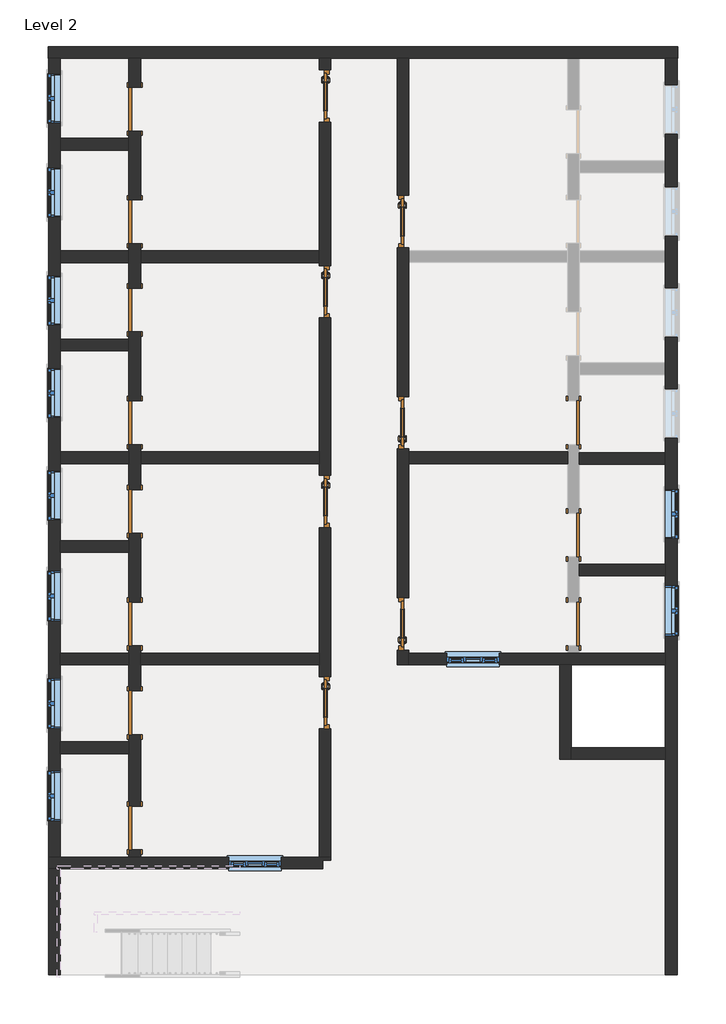
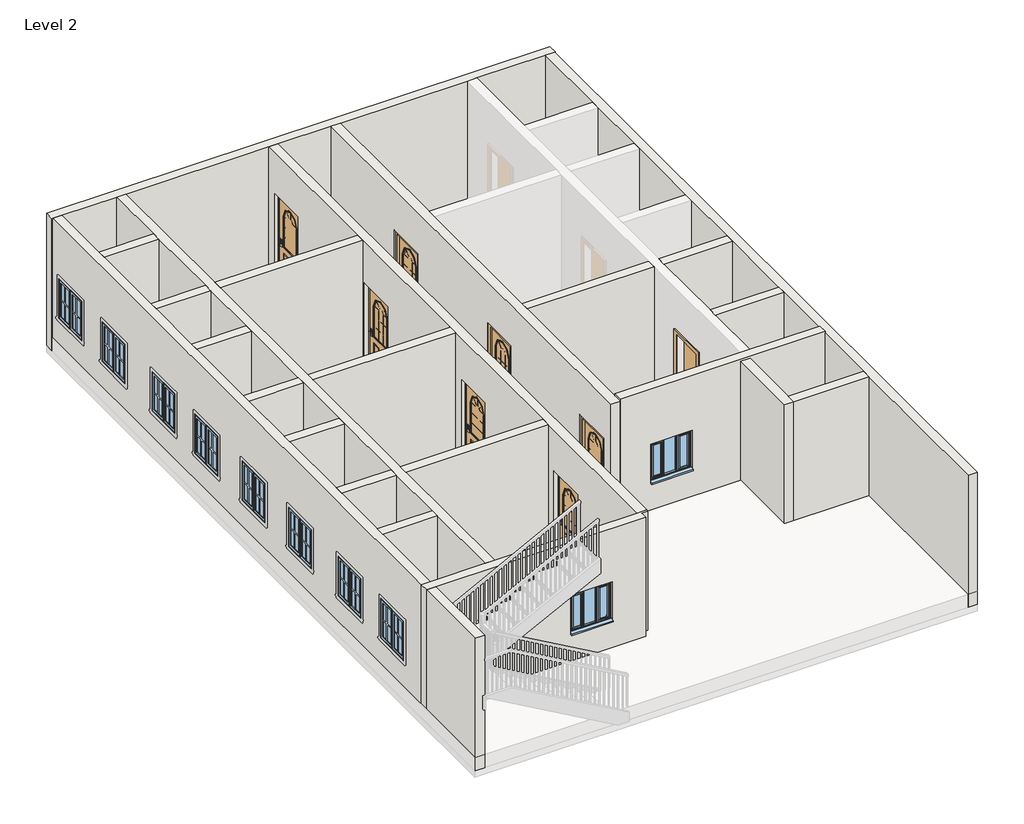
# One storey, part 1 of 4: 24 walls, 18 doors, 12 windows.
# Revit data of these elements (continued)
# Element 43 (IfcWindow, "Window-Casement-Double : 34\" x 36\"")
#   Mark = "17"
#   Window Inset = 0' - 0"
#   Interior Wall Closure = 0' - 2 1/4"
#   Frame Extension = 0' - 0 1/4"
#   Exterior Wall Closure = 0' - 1 1/4"
#   Interior Trim Visibility = yes
#   Exterior Trim Visibility = yes
#   Phase Created = New Construction
#   Materials on its faces: "Wood - Stained", "Glass", "Clad - White"
# Element 44 (IfcWindow, "Window-Casement-Double : 34\" x 36\"")
#   Mark = "18"
#   Window Inset = 0' - 0"
#   Interior Wall Closure = 0' - 2 1/4"
#   Frame Extension = 0' - 0 1/4"
#   Exterior Wall Closure = 0' - 1 1/4"
#   Interior Trim Visibility = yes
#   Exterior Trim Visibility = yes
#   Phase Created = New Construction
#   Materials on its faces: "Wood - Stained", "Glass", "Clad - White"
# Element 45 (IfcWindow, "Window-Casement-Double : 34\" x 36\"")
#   Mark = "19"
#   Window Inset = 0' - 0"
#   Interior Wall Closure = 0' - 2 1/4"
#   Frame Extension = 0' - 0 1/4"
#   Exterior Wall Closure = 0' - 1 1/4"
#   Interior Trim Visibility = yes
#   Exterior Trim Visibility = yes
#   Phase Created = New Construction
#   Materials on its faces: "Wood - Stained", "Glass", "Clad - White"
# Element 46 (IfcWindow, "Window-Casement-Double : 34\" x 36\"")
#   Mark = "20"
#   Window Inset = 0' - 0"
#   Interior Wall Closure = 0' - 2 1/4"
#   Frame Extension = 0' - 0 1/4"
#   Exterior Wall Closure = 0' - 1 1/4"
#   Interior Trim Visibility = yes
#   Exterior Trim Visibility = yes
#   Phase Created = New Construction
#   Materials on its faces: "Wood - Stained", "Glass", "Clad - White"
# Element 47 (IfcWindow, "Window-Casement-Double : 34\" x 36\"")
#   Mark = "21"
#   Window Inset = 0' - 0"
#   Interior Wall Closure = 0' - 2 1/4"
#   Frame Extension = 0' - 0 1/4"
#   Exterior Wall Closure = 0' - 1 1/4"
#   Interior Trim Visibility = yes
#   Exterior Trim Visibility = yes
#   Phase Created = New Construction
#   Materials on its faces: "Wood - Stained", "Glass", "Clad - White"
# Element 48 (IfcWindow, "Window-Casement-Double : 34\" x 36\"")
#   Mark = "22"
#   Window Inset = 0' - 0"
#   Interior Wall Closure = 0' - 2 1/4"
#   Frame Extension = 0' - 0 1/4"
#   Exterior Wall Closure = 0' - 1 1/4"
#   Interior Trim Visibility = yes
#   Exterior Trim Visibility = yes
#   Phase Created = New Construction
#   Materials on its faces: "Wood - Stained", "Glass", "Clad - White"
# Element 49 (IfcWindow, "Window-Casement-Double : 34\" x 36\"")
#   Mark = "23"
#   Window Inset = 0' - 0"
#   Interior Wall Closure = 0' - 2 1/4"
#   Frame Extension = 0' - 0 1/4"
#   Exterior Wall Closure = 0' - 1 1/4"
#   Interior Trim Visibility = yes
#   Exterior Trim Visibility = yes
#   Phase Created = New Construction
#   Materials on its faces: "Wood - Stained", "Glass", "Clad - White"
# Element 50 (IfcWindow, "Window-Casement-Double : 34\" x 36\"")
#   Mark = "24"
#   Window Inset = 0' - 0"
#   Interior Wall Closure = 0' - 2 1/4"
#   Frame Extension = 0' - 0 1/4"
#   Exterior Wall Closure = 0' - 1 1/4"
#   Interior Trim Visibility = yes
#   Exterior Trim Visibility = yes
#   Phase Created = New Construction
#   Materials on its faces: "Wood - Stained", "Glass", "Clad - White"
# Element 51 (IfcWindow, "Window-Casement-Double : 34\" x 36\"")
#   Mark = "25"
#   Window Inset = 0' - 0"
#   Interior Wall Closure = 0' - 2 1/4"
#   Frame Extension = 0' - 0 1/4"
#   Exterior Wall Closure = 0' - 1 1/4"
#   Interior Trim Visibility = yes
#   Exterior Trim Visibility = yes
#   Phase Created = New Construction
#   Materials on its faces: "Wood - Stained", "Glass", "Clad - White"
# Element 52 (IfcWindow, "Window-Casement-Double : 34\" x 36\"")
#   Mark = "26"
#   Window Inset = 0' - 0"
#   Interior Wall Closure = 0' - 2 1/4"
#   Frame Extension = 0' - 0 1/4"
#   Exterior Wall Closure = 0' - 1 1/4"
#   Interior Trim Visibility = yes
#   Exterior Trim Visibility = yes
#   Phase Created = New Construction
#   Materials on its faces: "Wood - Stained", "Glass", "Clad - White"
# Element 53 (IfcWindow, "Windows_Tpl_Plain : 910x910mm")
#   Mark = "31"
#   Phase Created = New Construction
#   Materials on its faces: "Window Frame", "Glass"
# Element 54 (IfcWindow, "Windows_Tpl_Plain : 910x910mm")
#   Mark = "32"
#   Phase Created = New Construction
#   Materials on its faces: "Window Frame", "Glass"
# Materials
#   "Door - Glazing": colour RGB 0 0 255, transparency 0.75
#   "Door - Panel": class "Wood", colour RGB 210 159 95, transparency 0, Cost = 0
#   "Door - Frame/Mullion": class "Wood", colour RGB 212 179 113, transparency 0
#   "Door - Handle": colour RGB 247 247 247, transparency 0
#   "Door - Frame": colour RGB 118 70 51, transparency 0, Cost = 0
#   "Wood - Stained": class "Wood", colour RGB 224 178 126, transparency 0, Cost = 0
#   "Glass": class "Glass", colour RGB 0 128 192, transparency 0.75, Description = "Soda Lime Glass", Cost = 0
#   "Clad - White": class "Wood", colour RGB 242 242 238, transparency 0, Cost = 0
#   "Window Frame": colour RGB 249 249 249, transparency 0
#   "Default Wall": colour RGB 128 128 128, transparency 0, Cost = 0
#   "Brick, Common": class "Masonry", colour RGB 170 98 104, transparency 0, Description = "Common brick", Cost = 0
#   "Doors - Glazing Bars": colour RGB 158 107 65, transparency 0
#   "Cherry": class "Wood", colour RGB 226 177 128, transparency 0, Description = "Prunus Serotina", Cost = 0
#   "Door - Architrave": class "Wood", colour RGB 154 90 5, transparency 0
#   "Earth": class "Generic", colour RGB 97 75 62, transparency 0, Description = "Soil", Cost = 0
